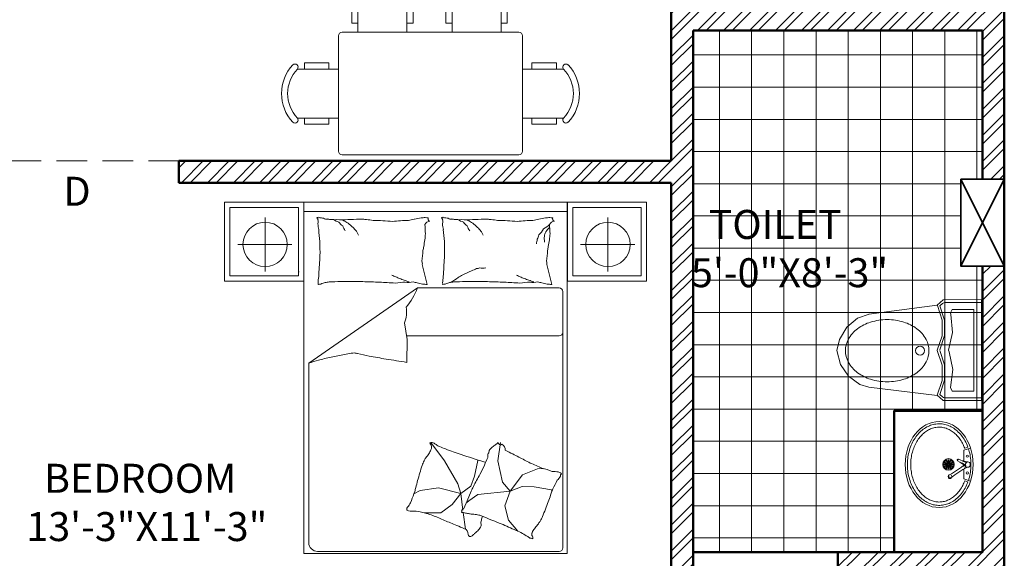
# Model space of a CAD drawing. Units: millimetres. Extents: x 67033 to 68301, y 155969 to 157209.
# Tile 3 of 17: x 67203 to 67407, y 156689 to 156800. Entities that reach past the tile are written whole.
import ezdxf

# ---------------------------------------------------------------- set-up
doc = ezdxf.new("R2010")
doc.units = ezdxf.units.MM
doc.linetypes.add('HIDDEN', pattern=[9.525, 6.35, -3.175])
for name, color, linetype, lineweight in [('A-ANNO-TEXT', 7, 'Continuous', 18), ('A-AREA-IDEN', 3, 'Continuous', 18), ('A-COLS', 3, 'Continuous', 35), ('A-FLOR-FIXT', 9, 'Continuous', 18), ('A-FLOR-OVHD', 1, 'HIDDEN', 18), ('A-FLOR-PATT', 252, 'Continuous', 13), ('A-FURN', 8, 'Continuous', 18), ('A-WALL', 7, 'Continuous', 50), ('A-WALL-PATT', 8, 'Continuous', 13)]:
    doc.layers.add(name, color=color, linetype=linetype, lineweight=lineweight)
doc.styles.add('DIM_FONT', font='SIMPLEX.shx', dxfattribs={"width": 0.8})
doc.styles.get("Standard").update_dxf_attribs({"font": 'arial.ttf'})

# ---------------------------------------------------------------- blocks, each defined once
blk = doc.blocks.new('A$C1AC47749')
for p, q in [((0.1857, 0.4482), (0.192, 0.4291)), ((0.1907, 0.471), (0.2068, 0.4222)), ((0.4293, 0.471), (0.4132, 0.4222)), ((0.4343, 0.4482), (0.428, 0.4291)), ((0.2068, 0.4222), (0.2842, 0.4222)), ((0.328, 0.4053), (0.3724, 0.3403)), ((0.4132, 0.4222), (0.3413, 0.4222)), ((0.3893, 0.3519), (0.3454, 0.4162))]:
    blk.add_line(p, q)
for centre, radius in [((0.2494, 0.448), 0.00831), ((0.3706, 0.448), 0.00831), ((0.3092, 0.3122), 0.0419), ((0.3092, 0.3122), 0.0344), ((0.3092, 0.3122), 0.00537)]:
    blk.add_circle(centre, radius)
for centre, radius, start, end in [((0.0375, 0.4868), 0.255, 336.13579, 352.27707), ((0.5085, 0.2596), 0.255, 136.21432, 152.3556), ((0.2063, 0.4499), 0.0866, 334.5047, 356.00596), ((0.31, 0.4499), 0.02, 316.21432, 172.27707), ((0.3092, 0.4498), 0.0162, 192.84427, 306.07085), ((0.3746, 0.3688), 0.0866, 132.48544, 153.98669), ((0.4278, 0.4728), 0.1, 191.02619, 214.5133), ((0.3603, 0.4414), 0.0293, 186.64626, 215.15328), ((0.2768, 0.381), 0.00664, 156.13579, 332.3556), ((0.2783, 0.3821), 0.00491, 187.76508, 270.74833), ((0.1778, 0.1242), 0.3257, 64.69826, 65.8021), ((0.2456, 0.3486), 0.1, 34.51324, 47.88111), ((0.299, 0.3998), 0.0293, 33.00691, 56.74915), ((0.29, 0.2836), 0.1, 20.01079, 34.51324), ((0.3971, 0.3226), 0.0139, 200.01079, 49.01574), ((0.3943, 0.3268), 0.00759, 93.32422, 152.57703), ((0.4717, 0.4086), 0.1, 214.5133, 229.01574), ((0.397, 0.323), 0.00812, 242.55567, 44.63645), ((0.3988, 0.322), 0.00965, 313.38275, 23.63796)]:
    blk.add_arc(centre, radius, start, end)
for centre, major_axis, ratio in [((0.31, 0.2449), (-0.31, 0), 0.790323), ((0.2894, 0.3122), (0.0145, 0), 0.137964), ((0.292, 0.3221), (0.0126, -0.0072), 0.137964), ((0.292, 0.3022), (0.0126, 0.0072), 0.137964), ((0.2993, 0.3294), (0.0072, -0.0126), 0.137964), ((0.2993, 0.295), (0.0072, 0.0126), 0.137964), ((0.3092, 0.332), (0, -0.0145), 0.137964), ((0.3092, 0.2923), (0, 0.0145), 0.137964), ((0.3192, 0.3294), (-0.0072, -0.0126), 0.137964), ((0.3192, 0.295), (-0.0072, 0.0126), 0.137964), ((0.3264, 0.3221), (-0.0126, -0.0072), 0.137964), ((0.3264, 0.3022), (-0.0126, 0.0072), 0.137964), ((0.3291, 0.3122), (-0.0145, 0), 0.137964)]:
    blk.add_ellipse(centre, major_axis=major_axis, ratio=ratio)
for points, knots in [([(0.1844, 0.4522), (0.1793, 0.4504), (0.1743, 0.4484), (0.1546, 0.44), (0.1406, 0.4328), (0.1143, 0.4165), (0.102, 0.4076), (0.0797, 0.3882), (0.0697, 0.3778), (0.052, 0.3558), (0.0443, 0.3443), (0.0317, 0.3205), (0.0267, 0.3083), (0.0194, 0.2833), (0.0171, 0.2706), (0.0158, 0.2536), (0.0156, 0.2492), (0.0156, 0.2449), (0.0156, 0.2369), (0.0162, 0.229), (0.019, 0.2084), (0.022, 0.1958), (0.0309, 0.1711), (0.0366, 0.159), (0.0508, 0.1357), (0.0591, 0.1244), (0.0781, 0.1031), (0.0888, 0.0931), (0.1123, 0.0746), (0.1251, 0.066), (0.1524, 0.0508), (0.1669, 0.0441), (0.1972, 0.0327), (0.213, 0.028), (0.2454, 0.0207), (0.262, 0.0182), (0.2956, 0.0154), (0.3125, 0.0152), (0.3462, 0.0169), (0.3629, 0.0189), (0.3956, 0.0251), (0.4117, 0.0293), (0.4426, 0.0397), (0.4574, 0.046), (0.4855, 0.0604), (0.4987, 0.0685), (0.5232, 0.0863), (0.5344, 0.096), (0.5545, 0.1167), (0.5635, 0.1277), (0.5788, 0.1506), (0.5851, 0.1625), (0.5953, 0.187), (0.599, 0.1995), (0.6037, 0.2248), (0.6047, 0.2375), (0.6039, 0.263), (0.6021, 0.2758), (0.5959, 0.3009), (0.5914, 0.3133), (0.5798, 0.3373), (0.5727, 0.349), (0.556, 0.3714), (0.5464, 0.382), (0.5249, 0.402), (0.5131, 0.4113), (0.4875, 0.4282), (0.4738, 0.4358), (0.4516, 0.446), (0.4437, 0.4492), (0.4356, 0.4522)], [5.14883, 5.14883, 5.14883, 5.14883, 5.205467, 5.205467, 5.375452, 5.375452, 5.545437, 5.545437, 5.715422, 5.715422, 5.885408, 5.885408, 6.055393, 6.055393, 6.225378, 6.225378, 6.283185, 6.283185, 6.283185, 6.389094, 6.389094, 6.559079, 6.559079, 6.729064, 6.729064, 6.89905, 6.89905, 7.069035, 7.069035, 7.23902, 7.23902, 7.409005, 7.409005, 7.578991, 7.578991, 7.748976, 7.748976, 7.918961, 7.918961, 8.088947, 8.088947, 8.258932, 8.258932, 8.428917, 8.428917, 8.598902, 8.598902, 8.768888, 8.768888, 8.938873, 8.938873, 9.108858, 9.108858, 9.278843, 9.278843, 9.448829, 9.448829, 9.618814, 9.618814, 9.788799, 9.788799, 9.958784, 9.958784, 10.12877, 10.12877, 10.298755, 10.298755, 10.46874, 10.46874, 10.559126, 10.559126, 10.559126, 10.559126]), ([(0.192, 0.4291), (0.1828, 0.4257), (0.1739, 0.4219), (0.1529, 0.4117), (0.1412, 0.4049), (0.1193, 0.3901), (0.1093, 0.382), (0.0911, 0.3649), (0.0829, 0.3558), (0.0687, 0.3371), (0.0626, 0.3273), (0.0526, 0.3074), (0.0487, 0.2972), (0.043, 0.2767), (0.0411, 0.2663), (0.0401, 0.2522), (0.04, 0.2486), (0.04, 0.2449), (0.04, 0.2369), (0.0406, 0.229), (0.0435, 0.2107), (0.0461, 0.2004), (0.0536, 0.1801), (0.0584, 0.1701), (0.0702, 0.1506), (0.0771, 0.1411), (0.093, 0.1229), (0.1019, 0.1142), (0.1217, 0.098), (0.1324, 0.0904), (0.1556, 0.0766), (0.168, 0.0704), (0.1939, 0.0596), (0.2075, 0.055), (0.2356, 0.0476), (0.2501, 0.0447), (0.2794, 0.0409), (0.2943, 0.0399), (0.3242, 0.0398), (0.3391, 0.0408), (0.3685, 0.0445), (0.3829, 0.0472), (0.4111, 0.0546), (0.4247, 0.0591), (0.4508, 0.0698), (0.4632, 0.076), (0.4864, 0.0897), (0.4973, 0.0972), (0.5171, 0.1134), (0.5262, 0.122), (0.5422, 0.1401), (0.5492, 0.1496), (0.561, 0.1691), (0.5659, 0.1791), (0.5736, 0.1994), (0.5763, 0.2097), (0.5797, 0.2304), (0.5803, 0.2408), (0.5794, 0.2617), (0.5779, 0.272), (0.5728, 0.2926), (0.5692, 0.3029), (0.5599, 0.3229), (0.5541, 0.3327), (0.5405, 0.3517), (0.5327, 0.3609), (0.5151, 0.3783), (0.5053, 0.3865), (0.4839, 0.4017), (0.4724, 0.4087), (0.4499, 0.4202), (0.4392, 0.4249), (0.428, 0.4291)], [5.15203, 5.15203, 5.15203, 5.15203, 5.262547, 5.262547, 5.423175, 5.423175, 5.583803, 5.583803, 5.744431, 5.744431, 5.90506, 5.90506, 6.065688, 6.065688, 6.226316, 6.226316, 6.283185, 6.283185, 6.283185, 6.405631, 6.405631, 6.566259, 6.566259, 6.726887, 6.726887, 6.887515, 6.887515, 7.048143, 7.048143, 7.208772, 7.208772, 7.3694, 7.3694, 7.530028, 7.530028, 7.690656, 7.690656, 7.851284, 7.851284, 8.011912, 8.011912, 8.172541, 8.172541, 8.333169, 8.333169, 8.493797, 8.493797, 8.654425, 8.654425, 8.815053, 8.815053, 8.975681, 8.975681, 9.13631, 9.13631, 9.296938, 9.296938, 9.457566, 9.457566, 9.618194, 9.618194, 9.778822, 9.778822, 9.93945, 9.93945, 10.100079, 10.100079, 10.260707, 10.260707, 10.421335, 10.421335, 10.555929, 10.555929, 10.555929, 10.555929]), ([(0.4244, 0.4561), (0.4209, 0.4573), (0.4174, 0.4584), (0.3981, 0.4641), (0.3818, 0.4677), (0.3487, 0.4726), (0.3319, 0.474), (0.2982, 0.4744), (0.2813, 0.4735), (0.248, 0.4694), (0.2315, 0.4663), (0.2088, 0.4603), (0.2022, 0.4583), (0.1956, 0.4561)], [4.3173628, 4.3173628, 4.3173628, 4.3173628, 4.3555402, 4.3555402, 4.5255255, 4.5255255, 4.6955107, 4.6955107, 4.865496, 4.865496, 5.0354813, 5.0354813, 5.1074083, 5.1074083, 5.1074083, 5.1074083])]:
    blk.add_open_spline(points, degree=3, knots=knots)
blk = doc.blocks.new('A$C09D638C3')
for p, q in [((0, 0.7166), (0.0008, 0.5263)), ((0.2504, 0.7166), (0, 0.7166)), ((0.0137, 0.7166), (0.0137, 0.5365)), ((0.2504, 0.7166), (0.5, 0.7166)), ((0.4871, 0.7166), (0.4871, 0.5365)), ((0.5, 0.7166), (0.5, 0.5263)), ((0.048, 0.6794), (0.048, 0.5712)), ((0.2504, 0.6794), (0.048, 0.6794)), ((0.2504, 0.6794), (0.4528, 0.6794)), ((0.4528, 0.6794), (0.4528, 0.5712)), ((0.048, 0.5712), (0.0652, 0.5632)), ((0.0733, 0.5655), (0.0652, 0.5632)), ((0.1631, 0.5735), (0.0733, 0.5655)), ((0.2504, 0.5527), (0.1631, 0.5735)), ((0.2582, 0.5558), (0.2504, 0.5527)), ((0.3462, 0.574), (0.2582, 0.5558)), ((0.4356, 0.5632), (0.3462, 0.574)), ((0.4528, 0.5712), (0.4356, 0.5632)), ((0.0008, 0.5263), (0.0274, 0.4973)), ((0.0137, 0.5365), (0.015, 0.5295)), ((0.015, 0.5295), (0.0189, 0.5233)), ((0.0189, 0.5233), (0.019, 0.5232)), ((0.019, 0.5232), (0.0309, 0.5105)), ((0.0271, 0.4967), (0.072, 0.1582)), ((0.0297, 0.4985), (0.0274, 0.4973)), ((0.102, 0.522), (0.0297, 0.4985)), ((0.1021, 0.5341), (0.0309, 0.5105)), ((0.1786, 0.5213), (0.102, 0.522)), ((0.1781, 0.5339), (0.1021, 0.5341)), ((0.2494, 0.5098), (0.1781, 0.5339)), ((0.2504, 0.4965), (0.1786, 0.5213)), ((0.2527, 0.4977), (0.2504, 0.4965)), ((0.3224, 0.5339), (0.2514, 0.5098)), ((0.3248, 0.5217), (0.2527, 0.4977)), ((0.3984, 0.5342), (0.3224, 0.5339)), ((0.4014, 0.5216), (0.3248, 0.5217)), ((0.47, 0.5105), (0.3984, 0.5342)), ((0.4734, 0.4973), (0.4014, 0.5216)), ((0.4758, 0.4967), (0.4334, 0.1581)), ((0.4818, 0.5232), (0.47, 0.5105)), ((0.5, 0.5263), (0.4734, 0.4973)), ((0.4818, 0.5232), (0.4857, 0.5293)), ((0.4857, 0.5293), (0.4871, 0.5363)), ((0.4871, 0.5363), (0.4871, 0.5365)), ((0.0718, 0.1596), (0.0917, 0.1021)), ((0.4201, 0.1144), (0.4334, 0.1581)), ((0.0917, 0.1021), (0.1359, 0.0488)), ((0.3799, 0.0583), (0.4201, 0.1144)), ((0.1359, 0.0488), (0.1968, 0.0131)), ((0.3218, 0.0186), (0.3799, 0.0583)), ((0.1968, 0.0131), (0.2526, 0)), ((0.2528, 0), (0.3218, 0.0186))]:
    blk.add_line(p, q)
blk.add_circle((0.2527, 0.4124), 0.0222)
for centre, radius, start, end in [((0.2776, 0.2962), 0.1668, 118.8748, 143.2661), ((0.2513, 0.3471), 0.1095, 89.1493, 119.7298), ((0.2546, 0.3471), 0.1095, 60.2702, 90.8507), ((0.2283, 0.2962), 0.1668, 36.7339, 61.1252), ((0.3216, 0.265), 0.2207, 143.6094, 162.4475), ((0.1843, 0.265), 0.2207, 17.5525, 36.3906), ((0.3937, 0.2468), 0.295, 163.3175, 179.5076), ((0.1122, 0.2468), 0.295, 0.4924, 16.6825), ((0.3937, 0.2519), 0.295, 180.4924, 196.6825), ((0.1122, 0.2519), 0.295, 343.3175, 359.5076), ((0.3216, 0.2338), 0.2207, 197.5525, 216.3906), ((0.1843, 0.2338), 0.2207, 323.6094, 342.4475), ((0.2776, 0.2026), 0.1668, 216.7339, 241.1252), ((0.2283, 0.2026), 0.1668, 298.8748, 323.2661), ((0.2513, 0.1516), 0.1095, 240.2702, 270.8507), ((0.2546, 0.1516), 0.1095, 269.1493, 299.7298)]:
    blk.add_arc(centre, radius, start, end)
blk = doc.blocks.new('A$C79766A75')
for p, q in [((0.45, 1.9999), (0, 1.9999)), ((0, 1.9999), (0, 1.5499)), ((0.42, 1.9699), (0.03, 1.9699)), ((0.03, 1.9699), (0.03, 1.5799)), ((0.42, 1.5799), (0.42, 1.9699)), ((0.45, 1.5499), (0.45, 1.9999)), ((1.9506, 2), (0.4506, 2)), ((0.4506, 2), (0.4506, 0)), ((1.9506, 0), (1.9506, 2)), ((2.402, 1.9999), (1.952, 1.9999)), ((1.952, 1.9999), (1.952, 1.5499)), ((2.372, 1.9699), (1.982, 1.9699)), ((1.982, 1.9699), (1.982, 1.5799)), ((2.372, 1.5799), (2.372, 1.9699)), ((2.402, 1.5499), (2.402, 1.9999)), ((0.2304, 1.9125), (0.2304, 1.6061)), ((1.9506, 1.9476), (0.4506, 1.9476)), ((2.1824, 1.9125), (2.1824, 1.6061)), ((0.0743, 1.7595), (0.3834, 1.7595)), ((2.0263, 1.7595), (2.3354, 1.7595)), ((1.1461, 1.5617), (1.1254, 1.6443)), ((1.8553, 1.5617), (1.8346, 1.6443)), ((0.03, 1.5799), (0.42, 1.5799)), ((0.4234, 1.6034), (0.4228, 1.6034)), ((1.982, 1.5799), (2.372, 1.5799)), ((0, 1.5499), (0.45, 1.5499)), ((1.1536, 1.5317), (1.1461, 1.5617)), ((1.8628, 1.5317), (1.8553, 1.5617)), ((1.952, 1.5499), (2.402, 1.5499)), ((1.0972, 1.5115), (0.4791, 1.0841)), ((1.0972, 1.5115), (1.9048, 1.5115)), ((1.9248, 1.4915), (1.9248, 0.0322)), ((1.0383, 1.2184), (1.0246, 1.3138)), ((1.9048, 1.2389), (1.0354, 1.2389)), ((1.0365, 1.0883), (1.0383, 1.2184)), ((0.4791, 0.0622), (0.4791, 1.0841)), ((1.1731, 0.6316), (1.2523, 0.5276)), ((1.5696, 0.6317), (1.5559, 0.5286)), ((1.2523, 0.5276), (1.3274, 0.3973)), ((1.4223, 0.4407), (1.442, 0.5296)), ((1.5559, 0.5286), (1.5817, 0.4065)), ((1.6952, 0.4478), (1.7898, 0.4856)), ((1.7898, 0.4856), (1.8139, 0.4822)), ((1.3274, 0.3973), (1.3452, 0.342)), ((1.4025, 0.3834), (1.4223, 0.4407)), ((1.5817, 0.4065), (1.6264, 0.355)), ((1.6264, 0.355), (1.6952, 0.4478)), ((1.1139, 0.3597), (1.0779, 0.3397)), ((1.2167, 0.3736), (1.1139, 0.3597)), ((1.3452, 0.342), (1.2167, 0.3736)), ((1.2957, 0.2787), (1.3452, 0.342)), ((1.3452, 0.342), (1.4025, 0.3834)), ((1.3452, 0.342), (1.3569, 0.2478)), ((1.4034, 0.3558), (1.3803, 0.2995)), ((1.6264, 0.355), (1.4406, 0.3361)), ((1.5954, 0.2725), (1.6264, 0.355)), ((1.6264, 0.355), (1.6935, 0.3825)), ((1.6935, 0.3825), (1.7623, 0.379)), ((1.7623, 0.379), (1.8603, 0.3619)), ((1.8603, 0.3619), (1.8636, 0.3554)), ((1.3803, 0.2995), (1.3626, 0.256)), ((1.3907, 0.3), (1.3787, 0.2914)), ((1.4406, 0.3361), (1.3907, 0.3)), ((1.1376, 0.2313), (1.2305, 0.2313)), ((1.2305, 0.2313), (1.2957, 0.2787)), ((1.3588, 0.2331), (1.3706, 0.1385)), ((1.6161, 0.19), (1.5954, 0.2725)), ((1.6697, 0.1274), (1.6161, 0.19)), ((1.9048, 0.0122), (0.5291, 0.0122)), ((0.4506, 0), (1.9506, 0))]:
    blk.add_line(p, q)
for centre in [(0.2304, 1.7595), (2.1824, 1.7595)]:
    blk.add_circle(centre, 0.126)
for centre, radius, start, end in [((0.5232, 1.9139), 0.00342, 291.7883, 340.436), ((0.525, 1.9085), 0.00232, 340.436, 101.8931), ((0.5246, 1.9378), 0.0251, 274.3025, 291.7883), ((0.5311, 1.9093), 0.00428, 201.9904, 281.8931), ((0.5486, 1.9393), 0.0289, 239.3487, 274.3025), ((0.5458, 1.8568), 0.0539, 59.3487, 84.7408), ((1.0352, 2.2041), 0.3048, 278.4372, 285.744), ((1.1179, 2.0719), 0.1611, 270, 278.4372), ((1.1592, 2.0011), 0.0904, 258.7276, 270), ((1.1709, 1.9049), 0.0131, 153.4195, 258.7276), ((1.2325, 1.9139), 0.00342, 291.7883, 340.436), ((1.2342, 1.9085), 0.00232, 340.436, 101.8931), ((1.2338, 1.9378), 0.0251, 274.3025, 291.7883), ((1.2404, 1.9093), 0.00428, 201.9904, 281.8931), ((1.2578, 1.9393), 0.0289, 239.3487, 274.3025), ((1.2551, 1.8568), 0.0539, 59.3487, 84.7408), ((1.7444, 2.2041), 0.3048, 278.4372, 285.744), ((1.8271, 2.0719), 0.1611, 270, 278.4372), ((1.8684, 2.0011), 0.0904, 258.7276, 270), ((1.8802, 1.9049), 0.0131, 153.4195, 258.7276), ((0.4996, 1.8889), 0.0328, 338.579, 8.1335), ((0.2896, 1.8253), 0.246, 8.1335, 12.1095), ((0.5465, 1.8994), 0.0156, 158.579, 201.9904), ((0.7297, 1.8867), 0.1983, 187.6809, 192.1095), ((0.546, 1.0829), 0.8208, 84.7408, 88.0921), ((0.6118, 2.0005), 0.0992, 254.0648, 274.2159), ((0.6775, 1.9817), 0.0992, 233.9136, 254.0648), ((0.6362, 0.406), 1.4943, 88.0921, 90.5757), ((0.7304, 1.9449), 0.0992, 216.1766, 233.9136), ((0.7737, 2.1075), 0.234, 242.7604, 249.1397), ((0.7661, 1.8961), 0.0992, 198.4397, 216.1766), ((0.7591, 1.0293), 0.8732, 90.5757, 94.8018), ((0.738, 1.949), 0.0768, 231.6114, 242.7604), ((0.974, 2.1633), 0.3916, 226.1885, 231.6114), ((0.9057, 1.9982), 0.2252, 219.0349, 226.1885), ((0.7631, 2.1919), 0.2897, 267.4614, 274.8018), ((0.8143, 2.0532), 0.1524, 259.8101, 267.4614), ((0.7515, 1.3747), 0.5293, 79.8101, 83.9133), ((0.8451, 0.8466), 1.049, 83.9133, 90), ((1.046, 1.2129), 0.6827, 90, 97.5469), ((1.1117, 1.6625), 0.2422, 97.5469, 105.744), ((1.171, 1.8579), 0.0342, 94.4002, 153.4195), ((1.6324, 1.8735), 0.4918, 180, 186.2324), ((1.2088, 1.8889), 0.0328, 338.579, 8.1335), ((0.9988, 1.8253), 0.246, 8.1335, 12.1095), ((1.2558, 1.8994), 0.0156, 158.579, 201.9904), ((1.4389, 1.8867), 0.1983, 187.6809, 192.1095), ((1.2552, 1.0829), 0.8208, 84.7408, 88.0921), ((1.3211, 2.0005), 0.0992, 254.0648, 274.2159), ((1.3868, 1.9817), 0.0992, 233.9136, 254.0648), ((1.3455, 0.406), 1.4943, 88.0921, 90.5757), ((1.4396, 1.9449), 0.0992, 216.1766, 233.9136), ((1.4829, 2.1075), 0.234, 242.7604, 249.1397), ((1.4753, 1.8961), 0.0992, 198.4397, 216.1766), ((1.4683, 1.0293), 0.8732, 90.5757, 94.8018), ((1.4473, 1.949), 0.0768, 231.6114, 242.7604), ((1.6833, 2.1633), 0.3916, 226.1885, 231.6114), ((1.615, 1.9982), 0.2252, 219.0349, 226.1885), ((1.4724, 2.1919), 0.2897, 267.4614, 274.8018), ((1.5236, 2.0532), 0.1524, 259.8101, 267.4614), ((1.4607, 1.3747), 0.5293, 79.8101, 83.9133), ((1.5543, 0.8466), 1.049, 83.9133, 90), ((1.7552, 1.2129), 0.6827, 90, 97.5469), ((1.821, 1.6625), 0.2422, 97.5469, 105.744), ((1.7511, 1.9723), 0.1399, 297.2036, 314.9024), ((1.784, 1.9167), 0.0899, 306.2641, 318.5571), ((1.8802, 1.8579), 0.0342, 94.4002, 153.4195), ((2.3416, 1.8735), 0.4918, 180, 186.2324), ((1.4472, 1.8987), 0.9131, 183.3687, 187.6809), ((0.7932, 1.8591), 0.0493, 208.3168, 219.0349), ((0.9392, 1.9062), 0.2002, 203.0028, 208.3168), ((1.3446, 1.7858), 0.204, 170.3156, 180), ((2.1565, 1.8987), 0.9131, 183.3687, 187.6809), ((1.5025, 1.8591), 0.0493, 208.3168, 219.0349), ((1.6484, 1.9062), 0.2002, 203.0028, 208.3168), ((1.6554, 1.8529), 0.1399, 332.6012, 343.485), ((1.6908, 1.9123), 0.1399, 314.9024, 332.6012), ((1.7653, 1.8132), 0.0562, 341.2201, 0), ((1.73, 1.7719), 0.0915, 0, 14.6851), ((1.6307, 1.8895), 0.2056, 338.1851, 341.2201), ((1.6887, 1.8881), 0.1511, 334.6449, 338.1851), ((1.7896, 1.8667), 0.0526, 318.5571, 334.6449), ((2.0538, 1.7858), 0.204, 170.3156, 180), ((1.2208, 1.7573), 0.6787, 178.3669, 183.3687), ((0.8192, 1.792), 0.3171, 347.8016, 351.9949), ((2.0027, 1.5994), 0.882, 167.8016, 170.3156), ((1.9301, 1.7573), 0.6787, 178.3669, 183.3687), ((1.6404, 1.8023), 0.1399, 343.485, 354.3689), ((1.5284, 1.792), 0.3171, 347.8016, 351.9949), ((2.7119, 1.5994), 0.882, 167.8016, 170.3156), ((14.1519, 0.85), 13.6356, 176.49514, 176.94504), ((1.9066, 1.6447), 1.3652, 176.945, 178.3669), ((0.4711, 1.7556), 0.6588, 351.9949, 357.3351), ((14.8612, 0.85), 13.6356, 176.49514, 176.94504), ((2.6158, 1.6447), 1.3652, 176.945, 178.3669), ((1.1803, 1.7556), 0.6588, 351.9949, 357.3351), ((1.0578, 1.6474), 0.0677, 357.3351, 14.0452), ((1.767, 1.6474), 0.0677, 357.3351, 14.0452), ((0.8521, 1.5209), 0.3212, 170.0016, 176.4951), ((0.6583, 0.9067), 0.7387, 64.6889, 66.5156), ((0.7015, 0.888), 0.7387, 66.5156, 68.3423), ((1.5613, 1.5209), 0.3212, 170.0016, 176.4951), ((0.9025, 2.1618), 0.7286, 302.135, 305.8263), ((1.1895, 1.8508), 0.3126, 296.4985, 302.135), ((0.7658, 2.8912), 1.4323, 294.3265, 296.4985), ((1.226, 2.0834), 0.5066, 290.6743, 294.3265), ((1.4305, 1.6796), 0.058, 274.0828, 290.6743), ((1.4679, 1.8969), 0.2721, 266.4448, 274.0828), ((1.3675, 0.9067), 0.7387, 64.6889, 66.5156), ((1.4107, 0.888), 0.7387, 66.5156, 68.3423), ((0.513, 1.535), 0.0193, 350.0016, 16.6978), ((0.5322, 1.5304), 0.00132, 16.6978, 97.1204), ((0.5579, 1.4467), 0.0875, 97.1204, 106.2212), ((0.5822, 1.4654), 0.0767, 106.2212, 117.2841), ((0.5507, 1.5832), 0.0453, 282.869, 297.2841), ((0.5623, 1.6885), 0.1459, 273.574, 282.869), ((0.589, 2.7103), 1.164, 270.2865, 273.574), ((0.7584, 7.2662), 5.7185, 269.0296, 270.2865), ((0.9401, 4.9065), 3.3622, 267.3904, 269.0296), ((0.9811, 2.7573), 1.2165, 265.3824, 267.3904), ((0.8583, 0.139), 1.4048, 85.3824, 87.2509), ((1.0175, 1.3138), 0.2301, 87.2509, 101.5586), ((0.7501, 0.8688), 0.7387, 68.3423, 70.572), ((0.8043, 0.8497), 0.7387, 70.572, 72.8018), ((1.0449, 1.6886), 0.1459, 263.5659, 281.5586), ((1.1099, 1.6599), 0.1197, 252.6136, 263.5659), ((1.0587, 1.3144), 0.2297, 72.6136, 80.5159), ((1.108, 1.2635), 0.2708, 80.5159, 85.9171), ((1.1535, 1.5308), 0.000917, 85.9171, 194.0449), ((1.2222, 1.535), 0.0193, 350.0016, 16.6978), ((1.2414, 1.5304), 0.00132, 16.6978, 97.1204), ((1.2671, 1.4467), 0.0875, 97.1204, 106.2212), ((1.2914, 1.4654), 0.0767, 106.2212, 117.2841), ((1.2599, 1.5832), 0.0453, 282.869, 297.2841), ((1.2716, 1.6885), 0.1459, 273.574, 282.869), ((1.2982, 2.7103), 1.164, 270.2865, 273.574), ((1.4677, 7.2662), 5.7185, 269.0296, 270.2865), ((1.6493, 4.9065), 3.3622, 267.3904, 269.0296), ((1.6903, 2.7573), 1.2165, 265.3824, 267.3904), ((1.5676, 0.139), 1.4048, 85.3824, 87.2509), ((1.7268, 1.3138), 0.2301, 87.2509, 101.5586), ((1.4594, 0.8688), 0.7387, 68.3423, 70.572), ((1.5136, 0.8497), 0.7387, 70.572, 72.8018), ((1.7541, 1.6886), 0.1459, 263.5659, 281.5586), ((1.8192, 1.6599), 0.1197, 252.6136, 263.5659), ((1.7679, 1.3144), 0.2297, 72.6136, 80.5159), ((1.8172, 1.2635), 0.2708, 80.5159, 85.9171), ((1.8627, 1.5308), 0.000917, 85.9171, 194.0449), ((0.745, 1.6407), 0.3751, 320.3555, 339.8512), ((1.9048, 1.4915), 0.02, 0, 90), ((0.8556, 1.3759), 0.1801, 339.8512, 8.1356), ((1.9048, 1.2589), 0.02, 270, 0), ((-0.1888, 5.1029), 4.0646, 280.7276, 282.9255), ((0.7282, 1.1989), 0.0581, 262.2696, 280.7276), ((0.7833, 1.3309), 0.1942, 256.8096, 262.2696), ((0.2481, -1.3253), 2.5158, 76.8096, 78.3259), ((0.3953, -1.4284), 2.588, 78.3259, 80.505), ((-0.0248, 2.8487), 1.8351, 285.9352, 287.7364), ((0.3872, 1.7415), 0.6574, 282.9255, 285.9352), ((0.413, -2.64), 3.7801, 80.505, 82.308), ((1.1752, 0.6267), 0.0063, 166.7192, 233.4208), ((1.1734, 0.6272), 0.00443, 93.9484, 166.7192), ((1.163, 0.6103), 0.0142, 10.4074, 53.4208), ((1.1755, 0.5964), 0.0352, 69.6548, 93.9484), ((1.1669, 0.5731), 0.0601, 51.4146, 69.6548), ((1.2538, 0.682), 0.0792, 231.4146, 247.2931), ((1.1426, 1.1456), 0.6605, 306.2163, 307.2151), ((1.7751, 0.3162), 0.3825, 126.2163, 127.5287), ((1.5806, 0.5924), 0.0452, 127.5287, 134.1274), ((1.5093, 0.6825), 0.0697, 308.8136, 314.1274), ((1.5706, 0.6318), 0.0127, 176.7545, 308.8136), ((1.5621, 0.59), 0.0359, 356.7545, 62.7098), ((0.9961, 0.6678), 0.194, 320.2995, 329.0944), ((0.8605, 0.749), 0.352, 329.0944, 333.1821), ((1.1396, 0.6079), 0.0393, 333.1821, 345.4291), ((1.1011, 0.5989), 0.0771, 2.7286, 10.4074), ((1.1628, 0.6019), 0.0153, 345.4291, 2.7286), ((1.5463, 1.3811), 0.8371, 247.2931, 249.8713), ((3.0113, 5.3783), 5.0942, 249.8713, 250.9164), ((2.374, 3.5362), 3.145, 250.9164, 253.3915), ((1.5435, 0.5526), 0.0458, 157.5838, 188.0492), ((1.4828, 0.5833), 0.0226, 324.1064, 8.0492), ((1.4519, 0.6426), 0.0774, 313.5224, 324.1064), ((1.383, 0.7705), 0.2176, 307.2151, 313.5224), ((0.2201, -2.1858), 3.0972, 62.7098, 63.5853), ((2.5711, 2.3551), 2.0162, 242.5001, 243.5853), ((1.3115, 0.4414), 0.1965, 153.9265, 162.1604), ((1.2077, 0.4922), 0.081, 140.2995, 153.9265), ((1.5084, 0.6341), 0.1166, 253.3915, 259.2634), ((2.4089, 0.1204), 1.0054, 154.9471, 157.5838), ((4.5245, 5.9445), 6.1019, 242.15178, 242.50014), ((-0.9881, -4.647), 5.8383, 62.15178, 62.50792), ((1.5182, -0.068), 0.6236, 62.5079, 69.2514), ((3.0311, -0.112), 2.003, 162.1604, 164.7375), ((2.8096, -0.3311), 1.5652, 150.064, 152.9116), ((2.9813, -0.2643), 1.6868, 152.9116, 154.9471), ((1.7121, 0.0657), 0.43, 69.2514, 77.3748), ((1.8682, 0.4049), 0.063, 77.3748, 93.3881), ((1.8955, 0.5247), 0.0599, 256.9598, 273.3881), ((1.9257, 0.5082), 0.0509, 238.3083, 256.9598), ((1.9279, 0.441), 0.0168, 130.5086, 180.9614), ((1.9201, 0.4587), 0.0058, 180.9614, 238.3083), ((2.6887, -0.0186), 1.6481, 164.7375, 166.159), ((-0.5166, 1.5491), 2.6619, 333.6668, 334.8268), ((1.8435, 0.4743), 0.0755, 310.5086, 333.6668), ((-1.4109, 1.284), 2.6619, 338.0627, 339.2227), ((0.9098, 0.4035), 0.1798, 339.2227, 343.6878), ((0.5589, 0.5062), 0.5454, 343.6878, 346.159), ((1.2176, 0.4627), 0.2143, 330.064, 337.7645), ((1.3456, 0.5261), 0.5454, 339.2919, 341.7631), ((1.701, 0.4319), 0.1798, 334.8268, 339.2919), ((0.9882, 0.3177), 0.0755, 314.9045, 338.0627), ((3.6966, -0.4634), 2.003, 157.7645, 160.3416), ((3.4079, -0.2212), 1.6481, 160.3416, 161.7631), ((1.0533, 0.2524), 0.0168, 134.9045, 185.3572), ((1.0424, 0.2513), 0.0058, 185.3572, 242.7041), ((1.0631, 0.2914), 0.0509, 242.7041, 261.3557), ((1.0645, 0.3003), 0.0599, 261.3557, 277.784), ((1.0811, 0.1786), 0.063, 81.7707, 97.784), ((1.0286, -0.1846), 0.43, 73.6473, 81.7707), ((0.974, -0.3705), 0.6236, 66.9038, 73.6473), ((1.3465, 0.2383), 0.00467, 287.1867, 70.6201), ((1.3486, 0.2247), 0.0092, 70.6201, 94.2593), ((1.3694, 0.234), 0.0231, 107.1867, 157.7645), ((1.3563, 0.267), 0.034, 262.0178, 274.2593), ((1.4091, 0.4221), 0.1955, 255.1193, 262.0178), ((1.358, 0.0507), 0.1794, 75.1193, 82.3216), ((1.4096, 0.153), 0.0712, 82.3216, 94.5118), ((-1.0716, -5.1672), 5.8383, 66.54766, 66.9038), ((3.6805, 5.7866), 6.1019, 246.54766, 246.89602), ((2.0773, 2.0287), 2.0162, 246.896, 247.9812), ((1.4285, 0.2893), 0.0663, 261.8784, 274.5118), ((1.4755, 0.332), 0.1166, 248.9957, 261.8784), ((2.7121, 3.1012), 3.145, 246.5205, 248.9957), ((1.505, 0.1766), 0.0458, 161.9797, 192.4451), ((2.4175, -0.1202), 1.0054, 160.6552, 161.9797), ((1.6279, 0.2819), 0.194, 315.9036, 324.6985), ((1.856, 0.1288), 0.081, 135.9036, 149.5306), ((1.9797, 0.1108), 0.1965, 149.5306, 157.7645), ((0.1602, -2.7118), 3.0972, 67.1056, 67.9812), ((1.3512, 0.1084), 0.0359, 1.1504, 67.1056), ((1.6722, -0.1762), 0.3825, 130.6122, 131.9246), ((0.9933, 0.6156), 0.6605, 310.6122, 311.611), ((1.2874, 0.2845), 0.2176, 311.611, 317.9183), ((1.3914, 0.1905), 0.0774, 317.9183, 328.5023), ((1.4382, 0.1619), 0.0226, 328.5023, 12.4451), ((3.6993, 4.7998), 5.0942, 245.4754, 246.5205), ((2.051, 0.8725), 0.8371, 242.8972, 245.4754), ((1.7345, 0.1188), 0.0153, 341.0332, 358.3327), ((1.6723, 0.1058), 0.0771, 358.3327, 6.0115), ((1.7162, 0.1388), 0.0393, 328.7862, 341.0332), ((1.4661, 0.3294), 0.352, 324.6985, 328.7862), ((0.5291, 0.0622), 0.05, 180, 270), ((1.3997, 0.1094), 0.0127, 181.1504, 313.2095), ((1.3607, 0.1509), 0.0697, 313.2095, 318.5233), ((1.4468, 0.0748), 0.0452, 131.9246, 138.5233), ((1.7576, 0.1689), 0.0792, 227.0187, 242.8972), ((1.6963, 0.0438), 0.0601, 47.0187, 65.2589), ((1.737, 0.0526), 0.0352, 65.2589, 89.5525), ((1.7401, 0.0928), 0.0142, 6.0115, 49.0249), ((1.756, 0.0832), 0.00443, 89.5525, 162.3233), ((1.7602, 0.0924), 0.0063, 162.3233, 229.0249), ((1.9048, 0.0322), 0.02, 270, 0)]:
    blk.add_arc(centre, radius, start, end)
at = {"style": 'DIM_FONT', "text_generation_flag": 4, "width": 0.8, "flags": 9}
for tag in ['XSIZE', 'YSIZE']:
    blk.add_attdef(tag, (1.9506, 2), '', height=0.0005, rotation=180, dxfattribs=at)
blk = doc.blocks.new('table dining')
for p, q in [((67480.1, 156784.21), (67480.1, 156775.8)), ((67490.26, 156775.8), (67490.26, 156784.21)), ((67499.62, 156784.21), (67499.62, 156775.8)), ((67509.78, 156775.8), (67509.78, 156784.21)), ((67480.1, 156782.75), (67478.83, 156782.75)), ((67478.83, 156777.67), (67478.83, 156782.75)), ((67490.26, 156782.75), (67491.53, 156782.75)), ((67491.53, 156777.67), (67491.53, 156782.75)), ((67499.62, 156782.75), (67498.35, 156782.75)), ((67498.35, 156777.67), (67498.35, 156782.75)), ((67509.78, 156782.75), (67511.05, 156782.75)), ((67511.05, 156777.67), (67511.05, 156782.75)), ((67480.1, 156777.67), (67478.83, 156777.67)), ((67490.26, 156777.67), (67491.53, 156777.67)), ((67499.62, 156777.67), (67498.35, 156777.67)), ((67509.78, 156777.67), (67511.05, 156777.67)), ((67476.09, 156751.17), (67476.09, 156775.04)), ((67476.85, 156775.8), (67513.43, 156775.8)), ((67514.19, 156751.17), (67514.19, 156775.04)), ((67476.09, 156768.18), (67467.57, 156768.18)), ((67469.03, 156768.18), (67469.03, 156769.45)), ((67474.11, 156769.45), (67469.03, 156769.45)), ((67474.11, 156768.18), (67474.11, 156769.45)), ((67514.19, 156768.18), (67522.71, 156768.18)), ((67516.16, 156768.18), (67516.16, 156769.45)), ((67516.16, 156769.45), (67521.24, 156769.45)), ((67521.24, 156768.18), (67521.24, 156769.45)), ((67467.57, 156758.02), (67476.09, 156758.02)), ((67469.03, 156758.02), (67469.03, 156756.75)), ((67474.11, 156758.02), (67474.11, 156756.75)), ((67522.71, 156758.02), (67514.19, 156758.02)), ((67516.16, 156758.02), (67516.16, 156756.75)), ((67521.24, 156758.02), (67521.24, 156756.75)), ((67474.11, 156756.75), (67469.03, 156756.75)), ((67516.16, 156756.75), (67521.24, 156756.75)), ((67476.85, 156750.4), (67513.43, 156750.4))]:
    blk.add_line(p, q)
for centre, radius, start, end in [((67485.18, 156778.87), 8.64, 46.4394, 133.5606), ((67485.18, 156778.87), 7.37, 46.4394, 133.5606), ((67504.7, 156778.87), 8.64, 46.4394, 133.5606), ((67504.7, 156778.87), 7.37, 46.4394, 133.5606), ((67479.7, 156784.71), 0.637, 138.3417, 308.7795), ((67490.66, 156784.71), 0.637, 231.2205, 41.6583), ((67499.22, 156784.71), 0.637, 138.3417, 308.7795), ((67510.18, 156784.71), 0.637, 231.2205, 41.6583), ((67476.85, 156775.04), 0.762, 90, 180), ((67513.43, 156775.04), 0.762, 0, 90), ((67472.91, 156763.1), 8.64, 136.4394, 223.5606), ((67472.91, 156763.1), 7.37, 136.4394, 223.5606), ((67467.07, 156768.58), 0.637, 321.2205, 131.6583), ((67523.2, 156768.58), 0.637, 48.3417, 218.7795), ((67517.37, 156763.1), 7.37, 316.4394, 43.5606), ((67517.37, 156763.1), 8.64, 316.4394, 43.5606), ((67467.07, 156757.62), 0.637, 228.3417, 38.7795), ((67523.2, 156757.62), 0.637, 141.2205, 311.6583), ((67476.85, 156751.17), 0.762, 180, 270), ((67513.43, 156751.17), 0.762, 270, 0)]:
    blk.add_arc(centre, radius, start, end)
blk = doc.blocks.new('COLUMN-230x460')
for p, q in [((0.44, 17.99), (9.44, -0.01)), ((9.44, 17.99), (0.44, -0.01))]:
    blk.add_line(p, q)
blk.add_lwpolyline([(0.44, 17.99), (9.44, 17.99), (9.44, -0.01), (0.44, -0.01)], close=True)

msp = doc.modelspace()

# ---------------------------------------------------------------- hatches: boundary and pattern name
at = {"layer": 'A-FLOR-PATT'}
h = msp.add_hatch(dxfattribs=at)
h.set_pattern_fill('NET', color=256, scale=2.1)
h.paths.add_polyline_path([(67402.94, 156797.99), (67342.94, 156797.99), (67342.94, 156689.99), (67372.94, 156689.99), (67384.62, 156689.99), (67384.62, 156719.26), (67402.94, 156719.26), (67402.94, 156749.19), (67398.44, 156749.19), (67398.44, 156767.19), (67402.94, 156767.19)])
h.paths.add_polyline_path([(67393.55, 156741.13), (67394.74, 156742.23), (67402.7, 156742.26), (67402.7, 156731.79), (67402.7, 156721.36), (67394.74, 156721.36), (67393.66, 156722.36), (67379.35, 156724.15), (67377.53, 156724.7), (67375.19, 156726.38), (67373.53, 156728.81), (67372.75, 156731.7), (67373.29, 156734.03), (67374.79, 156736.58), (67377.01, 156738.43), (67379.42, 156739.26)], flags=16)
h.paths.add_polyline_path([(67383.17, 156738.13, -0.07076), (67386.6, 156737.62, -0.082382), (67389.29, 156736.25, -0.106831), (67391.23, 156734.03, -0.13423), (67391.83, 156731.69, -0.13423), (67391.23, 156729.35, -0.106831), (67389.29, 156727.13, -0.082382), (67386.6, 156725.76, -0.07076), (67383.17, 156725.24, -0.07076), (67379.74, 156725.76, -0.082382), (67377.04, 156727.13, -0.106831), (67375.11, 156729.35, -0.13423), (67374.51, 156731.69, -0.13423), (67375.11, 156734.03, -0.106831), (67377.04, 156736.25, -0.082382), (67379.74, 156737.62, -0.07076)], flags=0)
h.paths.add_polyline_path([(67393.51, 156731.82), (67393.55, 156731.7), (67393.5, 156731.79)], flags=0)
h.paths.add_polyline_path([(67394.88, 156741.63), (67394.62, 156741.47), (67394.61, 156741.46), (67394.08, 156740.97), (67395.07, 156737.99), (67395.06, 156734.82), (67394.04, 156731.79), (67395.06, 156728.78), (67395.07, 156725.61), (67394.08, 156722.62), (67394.61, 156722.12), (67394.87, 156721.96), (67395.16, 156721.9), (67395.17, 156721.9), (67394.96, 156721.9), (67394.61, 156722.12), (67394.08, 156722.62), (67395.07, 156725.61), (67395.06, 156728.78), (67394.04, 156731.79), (67395.06, 156734.82), (67395.07, 156737.99), (67394.08, 156740.97), (67394.77, 156741.61)], flags=0)
h.paths.add_polyline_path([(67396.62, 156740.25), (67401.14, 156740.25), (67401.14, 156731.79), (67401.14, 156723.34), (67396.62, 156723.34), (67396.29, 156724.05), (67396.73, 156727.79), (67395.98, 156731.47), (67395.85, 156731.79), (67396.71, 156735.44), (67396.38, 156739.2), (67396.29, 156739.54)], flags=0)
h.paths.add_polyline_path([(67390.91, 156731.7, -1), (67389.06, 156731.7, -1)], flags=0)
h = msp.add_hatch(dxfattribs=at)
h.set_pattern_fill('NET', color=256, scale=2.1)
h.paths.add_polyline_path([(67393.55, 156741.13), (67394.74, 156742.23), (67402.7, 156742.26), (67402.7, 156731.79), (67402.7, 156721.36), (67394.74, 156721.36), (67393.66, 156722.36), (67379.35, 156724.15), (67377.53, 156724.7), (67375.19, 156726.38), (67373.53, 156728.81), (67372.75, 156731.7), (67373.29, 156734.03), (67374.79, 156736.58), (67377.01, 156738.43), (67379.42, 156739.26)], flags=16)
h.paths.add_polyline_path([(67330.02, 156741.43), (67385.97, 156741.43), (67385.97, 156763.82), (67330.02, 156763.82)], flags=9)
at = {"layer": 'A-WALL-PATT'}
h = msp.add_hatch(dxfattribs=at)
h.set_pattern_fill('ANSI32', color=256, scale=0.4)
h.paths.add_polyline_path([(67407.44, 156941.99), (67402.94, 156941.99), (67402.94, 156802.49), (67342.94, 156802.49), (67342.94, 156822.09), (67342.94, 156871.49), (67338.44, 156871.49), (67338.44, 156770.99), (67236.44, 156770.99), (67236.44, 156766.49), (67338.44, 156766.49), (67338.44, 156685.49), (67342.94, 156685.49), (67342.94, 156797.99), (67402.94, 156797.99), (67402.94, 156767.19), (67407.44, 156767.19)])
h = msp.add_hatch(dxfattribs=at)
h.set_pattern_fill('ANSI32', color=256, scale=0.4)
h.paths.add_polyline_path([(67407.44, 156749.19), (67402.94, 156749.19), (67402.94, 156689.99), (67384.62, 156689.99), (67372.94, 156689.99), (67372.94, 156685.49), (67402.94, 156685.49), (67402.94, 156640.49), (67407.44, 156640.49)])

# ---------------------------------------------------------------- linework, layer by layer
at = {"layer": 'A-FLOR-OVHD'}
msp.add_line((67236.44, 156770.99), (67196.98, 156770.99), dxfattribs=at)
at = {"layer": 'A-WALL'}
for p, q in [((67407.44, 157140.99), (67407.44, 156527.99)), ((67338.44, 156871.49), (67338.44, 156770.99)), ((67342.94, 156797.99), (67402.94, 156797.99)), ((67342.94, 156797.99), (67342.94, 156685.49)), ((67402.94, 156797.99), (67402.94, 156767.19)), ((67236.44, 156770.99), (67236.44, 156766.49)), ((67236.44, 156770.99), (67338.44, 156770.99)), ((67236.44, 156766.49), (67338.44, 156766.49)), ((67338.44, 156766.49), (67338.44, 156685.49)), ((67402.94, 156749.19), (67402.94, 156689.99)), ((67372.94, 156689.99), (67342.94, 156689.99)), ((67372.94, 156689.99), (67402.94, 156689.99)), ((67372.94, 156689.99), (67372.94, 156685.49))]:
    msp.add_line(p, q, dxfattribs=at)
msp.add_lwpolyline([(67402.94, 156719.26), (67384.62, 156719.26), (67384.62, 156689.99), (67402.94, 156689.99)], close=True, dxfattribs=at)

# ---------------------------------------------------------------- block references
at = {"layer": 'A-COLS'}
msp.add_blockref('COLUMN-230x460', (67398, 156749.2), dxfattribs=at)
at = {"layer": 'A-FLOR-FIXT', "rotation": 270}
for name, p, xscale, yscale, zscale in [('A$C09D638C3', (67372.75, 156742.26), 41.79230271587537, 41.79230271587537, 41.79230271587537), ('A$C1AC47749', (67386.91, 156717), 28.71035709425095, 28.71035709425095, 28.71035709425095)]:
    msp.add_blockref(name, p, dxfattribs=dict(at, xscale=xscale, yscale=yscale, zscale=zscale))
at = {"layer": 'A-FURN'}
msp.add_blockref('table dining', (-206.59, 21.85), dxfattribs=at)
at = {"layer": 'A-FURN', "xscale": 36.39326745080975, "yscale": 36.39326745080975, "zscale": 36.39326745080975}
msp.add_blockref('A$C79766A75', (67245.9, 156689.67), dxfattribs=at)

# ---------------------------------------------------------------- texts
at = {"layer": 'A-ANNO-TEXT', "insert": (67207.01, 156767.71), "char_height": 6, "attachment_point": 1}
msp.add_mtext_dynamic_manual_height_columns('   D', width=19.5287, gutter_width=12.5, heights=[0], dxfattribs=at)
at = {"layer": 'A-AREA-IDEN', "char_height": 6, "attachment_point": 1}
for s, width, insert in [('        TOILET\\P      5\'-0"X8\'-3"', 75.351, (67331.52, 156760.84)), ('  BEDROOM \\P13\'-3"X11\'-3"', 59.4046, (67204.81, 156708.26))]:
    msp.add_mtext_dynamic_manual_height_columns(s, width=width, gutter_width=12.5, heights=[0], dxfattribs=dict(at, insert=insert))

doc.saveas('drawing.dxf')
